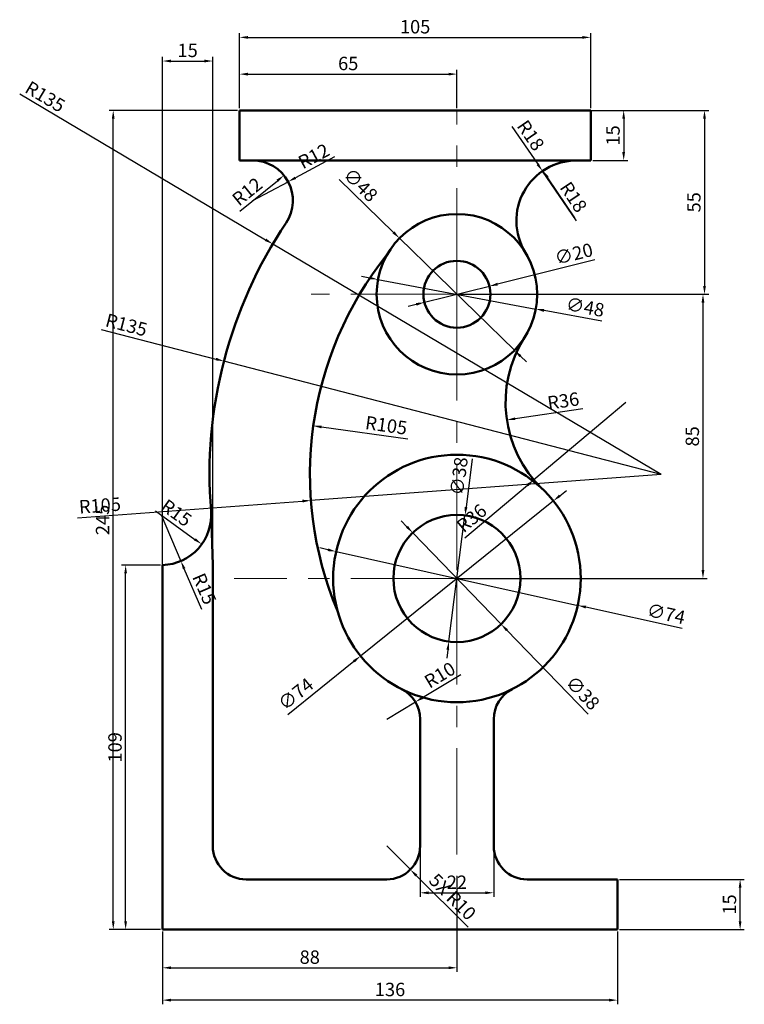
# Model space of a CAD drawing. Units: millimetres. Extents: x 3315 to 3532, y 1569 to 1864.
import ezdxf

# ---------------------------------------------------------------- set-up
doc = ezdxf.new("R2010")
doc.units = ezdxf.units.MM
doc.linetypes.add('CENTER', pattern=[50.8, 31.75, -6.35, 6.35, -6.35])
for name, color, linetype, lineweight in [('M-CNTR', 2, 'CENTER', 18), ('M-DIMS', 120, 'Continuous', 25), ('M-OUTL', 7, 'Continuous', 50)]:
    doc.layers.add(name, color=color, linetype=linetype, lineweight=lineweight)
doc.styles.get("Standard").update_dxf_attribs({"font": 'arial.ttf'})
doc.dimstyles.new('ISO-25', dxfattribs={"dimtxt": 4, "dimasz": 2.5, "dimexe": 1.25, "dimexo": 0.625, "dimtad": 1, "dimtxsty": 'Standard', "dimcen": 2.5, "dimadec": 0, "dimazin": 0, "dimtfac": 1, "dimtmove": 0, "dimatfit": 3, "dimfxl": 1, "dimarcsym": 0})

# ---------------------------------------------------------------- blocks, each defined once
blk = doc.blocks.new('*D1')
at = {"layer": 'Defpoints', "color": 0, "transparency": 16777216}
for p in [(3485.59, 1858.49), (3380.59, 1836.66), (3485.59, 1836.66)]:
    blk.add_point(p, dxfattribs=at)
at = {"layer": 'M-DIMS', "color": 0, "lineweight": -2, "transparency": 16777216}
for p, q in [((3380.59, 1837.28), (3380.59, 1859.74)), ((3383.09, 1858.49), (3483.09, 1858.49)), ((3485.59, 1837.28), (3485.59, 1859.74))]:
    blk.add_line(p, q, dxfattribs=at)
at = {"layer": 'M-DIMS', "color": 0, "transparency": 16777216}
for points in [[(3383.09, 1858.9), (3383.09, 1858.07), (3380.59, 1858.49)], [(3483.09, 1858.9), (3483.09, 1858.07), (3485.59, 1858.49)]]:
    blk.add_solid(points, dxfattribs=at)
at = {"layer": 'M-DIMS', "color": 0, "transparency": 16777216, "insert": (3433.09, 1861.15), "char_height": 4, "attachment_point": 5}
blk.add_mtext('105', dxfattribs=at)
blk = doc.blocks.new('*D2')
at = {"layer": 'Defpoints', "color": 0, "transparency": 16777216}
for p in [(3445.59, 1847.5), (3380.59, 1836.66), (3445.59, 1836.66)]:
    blk.add_point(p, dxfattribs=at)
at = {"layer": 'M-DIMS', "color": 0, "lineweight": -2, "transparency": 16777216}
for p, q in [((3380.59, 1837.28), (3380.59, 1848.75)), ((3383.09, 1847.5), (3443.09, 1847.5)), ((3445.59, 1837.28), (3445.59, 1848.75))]:
    blk.add_line(p, q, dxfattribs=at)
at = {"layer": 'M-DIMS', "color": 0, "transparency": 16777216}
for points in [[(3383.09, 1847.91), (3383.09, 1847.08), (3380.59, 1847.5)], [(3443.09, 1847.91), (3443.09, 1847.08), (3445.59, 1847.5)]]:
    blk.add_solid(points, dxfattribs=at)
at = {"layer": 'M-DIMS', "color": 0, "transparency": 16777216, "insert": (3413.09, 1850.16), "char_height": 4, "attachment_point": 5}
blk.add_mtext('65', dxfattribs=at)
blk = doc.blocks.new('*D3')
at = {"layer": 'Defpoints', "color": 0, "transparency": 16777216}
for p in [(3485.59, 1836.66), (3485.59, 1821.66), (3495.44, 1821.66)]:
    blk.add_point(p, dxfattribs=at)
at = {"layer": 'M-DIMS', "color": 0, "lineweight": -2, "transparency": 16777216}
for p, q in [((3486.21, 1836.66), (3496.69, 1836.66)), ((3495.44, 1834.16), (3495.44, 1824.16)), ((3486.21, 1821.66), (3496.69, 1821.66))]:
    blk.add_line(p, q, dxfattribs=at)
at = {"layer": 'M-DIMS', "color": 0, "transparency": 16777216}
for points in [[(3495.02, 1834.16), (3495.85, 1834.16), (3495.44, 1836.66)], [(3495.02, 1824.16), (3495.85, 1824.16), (3495.44, 1821.66)]]:
    blk.add_solid(points, dxfattribs=at)
at = {"layer": 'M-DIMS', "color": 0, "transparency": 16777216, "insert": (3492.77, 1829.16), "char_height": 4, "attachment_point": 5, "rotation": 90}
blk.add_mtext('15', dxfattribs=at)
blk = doc.blocks.new('*D4')
at = {"layer": 'Defpoints', "color": 0, "transparency": 16777216}
for p in [(3445.59, 1836.66), (3445.59, 1781.66), (3519.6, 1781.66)]:
    blk.add_point(p, dxfattribs=at)
at = {"layer": 'M-DIMS', "color": 0, "lineweight": -2, "transparency": 16777216}
for p, q in [((3446.21, 1836.66), (3520.85, 1836.66)), ((3519.6, 1834.16), (3519.6, 1784.16)), ((3446.21, 1781.66), (3520.85, 1781.66))]:
    blk.add_line(p, q, dxfattribs=at)
at = {"layer": 'M-DIMS', "color": 0, "transparency": 16777216}
for points in [[(3519.18, 1834.16), (3520.02, 1834.16), (3519.6, 1836.66)], [(3519.18, 1784.16), (3520.02, 1784.16), (3519.6, 1781.66)]]:
    blk.add_solid(points, dxfattribs=at)
at = {"layer": 'M-DIMS', "color": 0, "transparency": 16777216, "insert": (3516.94, 1809.16), "char_height": 4, "attachment_point": 5, "rotation": 90}
blk.add_mtext('55', dxfattribs=at)
blk = doc.blocks.new('*D5')
at = {"layer": 'Defpoints', "color": 0, "transparency": 16777216}
for p in [(3445.59, 1781.66), (3445.59, 1696.66), (3519.15, 1696.66)]:
    blk.add_point(p, dxfattribs=at)
at = {"layer": 'M-DIMS', "color": 0, "lineweight": -2, "transparency": 16777216}
for p, q in [((3446.21, 1781.66), (3520.4, 1781.66)), ((3519.15, 1779.16), (3519.15, 1699.16)), ((3446.21, 1696.66), (3520.4, 1696.66))]:
    blk.add_line(p, q, dxfattribs=at)
at = {"layer": 'M-DIMS', "color": 0, "transparency": 16777216}
for points in [[(3518.73, 1779.16), (3519.57, 1779.16), (3519.15, 1781.66)], [(3518.73, 1699.16), (3519.57, 1699.16), (3519.15, 1696.66)]]:
    blk.add_solid(points, dxfattribs=at)
at = {"layer": 'M-DIMS', "color": 0, "transparency": 16777216, "insert": (3516.48, 1739.16), "char_height": 4, "attachment_point": 5, "rotation": 90}
blk.add_mtext('85', dxfattribs=at)
blk = doc.blocks.new('*D6')
at = {"layer": 'Defpoints', "color": 0, "transparency": 16777216}
for p in [(3434.59, 1635.64), (3456.59, 1635.64), (3456.59, 1602.65)]:
    blk.add_point(p, dxfattribs=at)
at = {"layer": 'M-DIMS', "color": 0, "lineweight": -2, "transparency": 16777216}
for p, q in [((3434.59, 1635.01), (3434.59, 1601.4)), ((3456.59, 1635.01), (3456.59, 1601.4)), ((3437.09, 1602.65), (3454.09, 1602.65))]:
    blk.add_line(p, q, dxfattribs=at)
at = {"layer": 'M-DIMS', "color": 0, "transparency": 16777216}
for points in [[(3437.09, 1603.07), (3437.09, 1602.24), (3434.59, 1602.65)], [(3454.09, 1603.07), (3454.09, 1602.24), (3456.59, 1602.65)]]:
    blk.add_solid(points, dxfattribs=at)
at = {"layer": 'M-DIMS', "color": 0, "transparency": 16777216, "insert": (3445.59, 1605.29), "char_height": 4, "attachment_point": 5}
blk.add_mtext('22', dxfattribs=at)
blk = doc.blocks.new('*D7')
at = {"layer": 'Defpoints', "color": 0, "transparency": 16777216}
for p in [(3357.59, 1591.66), (3493.59, 1591.66), (3357.59, 1570.55)]:
    blk.add_point(p, dxfattribs=at)
at = {"layer": 'M-DIMS', "color": 0, "lineweight": -2, "transparency": 16777216}
for p, q in [((3357.59, 1591.03), (3357.59, 1569.3)), ((3493.59, 1591.03), (3493.59, 1569.3)), ((3491.09, 1570.55), (3360.09, 1570.55))]:
    blk.add_line(p, q, dxfattribs=at)
at = {"layer": 'M-DIMS', "color": 0, "transparency": 16777216}
for points in [[(3360.09, 1570.97), (3360.09, 1570.13), (3357.59, 1570.55)], [(3491.09, 1570.97), (3491.09, 1570.13), (3493.59, 1570.55)]]:
    blk.add_solid(points, dxfattribs=at)
at = {"layer": 'M-DIMS', "color": 0, "transparency": 16777216, "insert": (3425.59, 1573.22), "char_height": 4, "attachment_point": 5}
blk.add_mtext('136', dxfattribs=at)
blk = doc.blocks.new('*D8')
at = {"layer": 'Defpoints', "color": 0, "transparency": 16777216}
for p in [(3445.59, 1608.3), (3357.59, 1591.66), (3445.59, 1580.22)]:
    blk.add_point(p, dxfattribs=at)
at = {"layer": 'M-DIMS', "color": 0, "lineweight": -2, "transparency": 16777216}
for p, q in [((3445.59, 1607.67), (3445.59, 1578.97)), ((3357.59, 1591.03), (3357.59, 1578.97)), ((3360.09, 1580.22), (3443.09, 1580.22))]:
    blk.add_line(p, q, dxfattribs=at)
at = {"layer": 'M-DIMS', "color": 0, "transparency": 16777216}
for points in [[(3360.09, 1580.64), (3360.09, 1579.81), (3357.59, 1580.22)], [(3443.09, 1580.64), (3443.09, 1579.81), (3445.59, 1580.22)]]:
    blk.add_solid(points, dxfattribs=at)
at = {"layer": 'M-DIMS', "color": 0, "transparency": 16777216, "insert": (3401.59, 1582.89), "char_height": 4, "attachment_point": 5}
blk.add_mtext('88', dxfattribs=at)
blk = doc.blocks.new('*D9')
at = {"layer": 'Defpoints', "color": 0, "transparency": 16777216}
for p in [(3346.54, 1700.66), (3357.59, 1700.66), (3357.59, 1591.66)]:
    blk.add_point(p, dxfattribs=at)
at = {"layer": 'M-DIMS', "color": 0, "lineweight": -2, "transparency": 16777216}
for p, q in [((3356.96, 1700.66), (3345.29, 1700.66)), ((3346.54, 1594.16), (3346.54, 1698.16)), ((3356.96, 1591.66), (3345.29, 1591.66))]:
    blk.add_line(p, q, dxfattribs=at)
at = {"layer": 'M-DIMS', "color": 0, "transparency": 16777216}
for points in [[(3346.13, 1698.16), (3346.96, 1698.16), (3346.54, 1700.66)], [(3346.13, 1594.16), (3346.96, 1594.16), (3346.54, 1591.66)]]:
    blk.add_solid(points, dxfattribs=at)
at = {"layer": 'M-DIMS', "color": 0, "transparency": 16777216, "insert": (3343.88, 1646.16), "char_height": 4, "attachment_point": 5, "rotation": 90}
blk.add_mtext('109', dxfattribs=at)
blk = doc.blocks.new('*D10')
at = {"layer": 'Defpoints', "color": 0, "transparency": 16777216}
for p in [(3471.33, 1818.6), (3481.36, 1803.66)]:
    blk.add_point(p, dxfattribs=at)
at = {"layer": 'M-DIMS', "color": 0, "lineweight": -2, "transparency": 16777216}
blk.add_line((3480.81, 1804.48), (3472.72, 1816.53), dxfattribs=at)
at = {"layer": 'M-DIMS', "color": 0, "transparency": 16777216}
blk.add_solid([(3473.07, 1816.76), (3472.38, 1816.3), (3471.33, 1818.6)], dxfattribs=at)
at = {"layer": 'M-DIMS', "color": 0, "transparency": 16777216, "insert": (3480.01, 1810.46), "char_height": 4, "attachment_point": 5, "rotation": 303.8767}
blk.add_mtext('R18', dxfattribs=at)
blk = doc.blocks.new('*D11')
at = {"layer": 'Defpoints', "color": 0, "transparency": 16777216}
for p in [(3393.86, 1817.2), (3384.53, 1809.66)]:
    blk.add_point(p, dxfattribs=at)
at = {"layer": 'M-DIMS', "color": 0, "lineweight": -2, "transparency": 16777216}
blk.add_line((3380.68, 1806.54), (3391.92, 1815.63), dxfattribs=at)
at = {"layer": 'M-DIMS', "color": 0, "transparency": 16777216}
blk.add_solid([(3391.66, 1815.96), (3392.18, 1815.31), (3393.86, 1817.2)], dxfattribs=at)
at = {"layer": 'M-DIMS', "color": 0, "transparency": 16777216, "insert": (3383.21, 1811.97), "char_height": 4, "attachment_point": 5, "rotation": 38.9548}
blk.add_mtext('R12', dxfattribs=at)
blk = doc.blocks.new('*D12')
at = {"layer": 'Defpoints', "color": 0, "transparency": 16777216}
for p in [(3375.94, 1761.65), (3506.63, 1727.79)]:
    blk.add_point(p, dxfattribs=at)
at = {"layer": 'M-DIMS', "color": 0, "lineweight": -2, "transparency": 16777216}
for p, q in [((3339.23, 1771.17), (3373.52, 1762.28)), ((3506.63, 1727.79), (3375.94, 1761.65))]:
    blk.add_line(p, q, dxfattribs=at)
at = {"layer": 'M-DIMS', "color": 0, "transparency": 16777216}
blk.add_solid([(3373.63, 1762.68), (3373.42, 1761.88), (3375.94, 1761.65)], dxfattribs=at)
at = {"layer": 'M-DIMS', "color": 0, "transparency": 16777216, "insert": (3346.65, 1772), "char_height": 4, "attachment_point": 5, "rotation": 345.4735}
blk.add_mtext('R135', dxfattribs=at)
blk = doc.blocks.new('*D13')
at = {"layer": 'Defpoints', "color": 0, "transparency": 16777216}
for p in [(3402.63, 1742.3), (3506.63, 1727.79)]:
    blk.add_point(p, dxfattribs=at)
at = {"layer": 'M-DIMS', "color": 0, "lineweight": -2, "transparency": 16777216}
blk.add_line((3430.93, 1738.36), (3405.11, 1741.96), dxfattribs=at)
at = {"layer": 'M-DIMS', "color": 0, "transparency": 16777216}
blk.add_solid([(3405.17, 1742.37), (3405.05, 1741.55), (3402.63, 1742.3)], dxfattribs=at)
at = {"layer": 'M-DIMS', "color": 0, "transparency": 16777216, "insert": (3424.39, 1741.96), "char_height": 4, "attachment_point": 5, "rotation": 352.055}
blk.add_mtext('R105', dxfattribs=at)
blk = doc.blocks.new('*D14')
at = {"layer": 'Defpoints', "color": 0, "transparency": 16777216}
for p in [(3496.13, 1749.33), (3460.52, 1744.06)]:
    blk.add_point(p, dxfattribs=at)
at = {"layer": 'M-DIMS', "color": 0, "lineweight": -2, "transparency": 16777216}
blk.add_line((3483.19, 1747.41), (3462.99, 1744.42), dxfattribs=at)
at = {"layer": 'M-DIMS', "color": 0, "transparency": 16777216}
blk.add_solid([(3462.93, 1744.84), (3463.05, 1744.01), (3460.52, 1744.06)], dxfattribs=at)
at = {"layer": 'M-DIMS', "color": 0, "transparency": 16777216, "insert": (3477.45, 1749.26), "char_height": 4, "attachment_point": 5, "rotation": 8.4211}
blk.add_mtext('R36', dxfattribs=at)
blk = doc.blocks.new('*D15')
at = {"layer": 'Defpoints', "color": 0, "transparency": 16777216}
for p in [(3433.18, 1659.73), (3424.59, 1654.61)]:
    blk.add_point(p, dxfattribs=at)
at = {"layer": 'M-DIMS', "color": 0, "lineweight": -2, "transparency": 16777216}
for p, q in [((3446.74, 1667.82), (3435.32, 1661.01)), ((3424.59, 1654.61), (3433.18, 1659.73))]:
    blk.add_line(p, q, dxfattribs=at)
at = {"layer": 'M-DIMS', "color": 0, "transparency": 16777216}
blk.add_solid([(3435.11, 1661.37), (3435.54, 1660.65), (3433.18, 1659.73)], dxfattribs=at)
at = {"layer": 'M-DIMS', "color": 0, "transparency": 16777216, "insert": (3440.74, 1667.35), "char_height": 4, "attachment_point": 5, "rotation": 30.7966}
blk.add_mtext('R10', dxfattribs=at)
blk = doc.blocks.new('*D16')
at = {"layer": 'Defpoints', "color": 0, "transparency": 16777216}
for p in [(3357.12, 1715.66), (3369.3, 1706.9)]:
    blk.add_point(p, dxfattribs=at)
at = {"layer": 'M-DIMS', "color": 0, "lineweight": -2, "transparency": 16777216}
blk.add_line((3355.46, 1716.85), (3367.27, 1708.36), dxfattribs=at)
at = {"layer": 'M-DIMS', "color": 0, "transparency": 16777216}
blk.add_solid([(3367.51, 1708.7), (3367.02, 1708.02), (3369.3, 1706.9)], dxfattribs=at)
at = {"layer": 'M-DIMS', "color": 0, "transparency": 16777216, "insert": (3361.42, 1715.85), "char_height": 4, "attachment_point": 5, "rotation": 324.2811}
blk.add_mtext('R15', dxfattribs=at)
blk = doc.blocks.new('*D17')
at = {"layer": 'Defpoints', "color": 0, "transparency": 16777216}
for p in [(3428.41, 1798.42), (3462.76, 1764.9)]:
    blk.add_point(p, dxfattribs=at)
at = {"layer": 'M-DIMS', "color": 0, "lineweight": -2, "transparency": 16777216}
for p, q in [((3410.42, 1815.97), (3426.62, 1800.17)), ((3462.76, 1764.9), (3428.41, 1798.42)), ((3464.55, 1763.15), (3466.34, 1761.41))]:
    blk.add_line(p, q, dxfattribs=at)
at = {"layer": 'M-DIMS', "color": 0, "transparency": 16777216}
for points in [[(3426.91, 1800.46), (3426.33, 1799.87), (3428.41, 1798.42)], [(3464.84, 1763.45), (3464.26, 1762.85), (3462.76, 1764.9)]]:
    blk.add_solid(points, dxfattribs=at)
at = {"layer": 'M-DIMS', "color": 0, "transparency": 16777216, "insert": (3416.42, 1814), "char_height": 4, "attachment_point": 5, "rotation": 315.7036}
blk.add_mtext('∅48', dxfattribs=at)
blk = doc.blocks.new('*D18')
at = {"layer": 'Defpoints', "color": 0, "transparency": 16777216}
for p in [(3455.29, 1784.07), (3435.88, 1779.25)]:
    blk.add_point(p, dxfattribs=at)
at = {"layer": 'M-DIMS', "color": 0, "lineweight": -2, "transparency": 16777216}
for p, q in [((3486.81, 1791.91), (3457.72, 1784.67)), ((3435.88, 1779.25), (3455.29, 1784.07)), ((3433.45, 1778.64), (3431.03, 1778.04))]:
    blk.add_line(p, q, dxfattribs=at)
at = {"layer": 'M-DIMS', "color": 0, "transparency": 16777216}
for points in [[(3457.62, 1785.08), (3457.82, 1784.27), (3455.29, 1784.07)], [(3433.35, 1779.05), (3433.56, 1778.24), (3435.88, 1779.25)]]:
    blk.add_solid(points, dxfattribs=at)
at = {"layer": 'M-DIMS', "color": 0, "transparency": 16777216, "insert": (3480.64, 1793.24), "char_height": 4, "attachment_point": 5, "rotation": 13.962}
blk.add_mtext('∅20', dxfattribs=at)
blk = doc.blocks.new('*D19')
at = {"layer": 'Defpoints', "color": 0, "transparency": 16777216}
for p in [(3432.38, 1710.32), (3458.79, 1682.99)]:
    blk.add_point(p, dxfattribs=at)
at = {"layer": 'M-DIMS', "color": 0, "lineweight": -2, "transparency": 16777216}
for p, q in [((3430.65, 1712.12), (3428.91, 1713.92)), ((3432.38, 1710.32), (3458.79, 1682.99)), ((3484.79, 1656.07), (3460.52, 1681.2))]:
    blk.add_line(p, q, dxfattribs=at)
at = {"layer": 'M-DIMS', "color": 0, "transparency": 16777216}
for points in [[(3430.95, 1712.41), (3430.35, 1711.83), (3432.38, 1710.32)], [(3460.82, 1681.49), (3460.22, 1680.91), (3458.79, 1682.99)]]:
    blk.add_solid(points, dxfattribs=at)
at = {"layer": 'M-DIMS', "color": 0, "transparency": 16777216, "insert": (3482.85, 1662.08), "char_height": 4, "attachment_point": 5, "rotation": 314.0096}
blk.add_mtext('∅38', dxfattribs=at)
blk = doc.blocks.new('*D20')
at = {"layer": 'Defpoints', "color": 0, "transparency": 16777216}
for p in [(3409.47, 1704.7), (3481.7, 1688.62)]:
    blk.add_point(p, dxfattribs=at)
at = {"layer": 'M-DIMS', "color": 0, "lineweight": -2, "transparency": 16777216}
for p, q in [((3407.03, 1705.24), (3404.59, 1705.79)), ((3409.47, 1704.7), (3481.7, 1688.62)), ((3512.93, 1681.66), (3484.14, 1688.07))]:
    blk.add_line(p, q, dxfattribs=at)
at = {"layer": 'M-DIMS', "color": 0, "transparency": 16777216}
for points in [[(3407.12, 1705.65), (3406.94, 1704.84), (3409.47, 1704.7)], [(3484.23, 1688.48), (3484.05, 1687.67), (3481.7, 1688.62)]]:
    blk.add_solid(points, dxfattribs=at)
at = {"layer": 'M-DIMS', "color": 0, "transparency": 16777216, "insert": (3508.01, 1685.61), "char_height": 4, "attachment_point": 5, "rotation": 347.4467}
blk.add_mtext('∅74', dxfattribs=at)
blk = doc.blocks.new('*D21')
at = {"layer": 'Defpoints', "color": 0, "transparency": 16777216}
for p in [(3342.84, 1836.66), (3380.59, 1836.66), (3357.59, 1591.66)]:
    blk.add_point(p, dxfattribs=at)
at = {"layer": 'M-DIMS', "color": 0, "lineweight": -2, "transparency": 16777216}
for p, q in [((3379.96, 1836.66), (3341.59, 1836.66)), ((3342.84, 1594.16), (3342.84, 1834.16)), ((3356.96, 1591.66), (3341.59, 1591.66))]:
    blk.add_line(p, q, dxfattribs=at)
at = {"layer": 'M-DIMS', "color": 0, "transparency": 16777216}
for points in [[(3342.42, 1834.16), (3343.25, 1834.16), (3342.84, 1836.66)], [(3342.42, 1594.16), (3343.25, 1594.16), (3342.84, 1591.66)]]:
    blk.add_solid(points, dxfattribs=at)
at = {"layer": 'M-DIMS', "color": 0, "transparency": 16777216, "insert": (3340.17, 1714.16), "char_height": 4, "attachment_point": 5, "rotation": 90}
blk.add_mtext('245', dxfattribs=at)
blk = doc.blocks.new('*D22')
at = {"layer": 'Defpoints', "color": 0, "transparency": 16777216}
for p in [(3493.59, 1606.66), (3530.25, 1606.66), (3493.59, 1591.66)]:
    blk.add_point(p, dxfattribs=at)
at = {"layer": 'M-DIMS', "color": 0, "lineweight": -2, "transparency": 16777216}
for p, q in [((3494.21, 1606.66), (3531.5, 1606.66)), ((3530.25, 1594.16), (3530.25, 1604.16)), ((3494.21, 1591.66), (3531.5, 1591.66))]:
    blk.add_line(p, q, dxfattribs=at)
at = {"layer": 'M-DIMS', "color": 0, "transparency": 16777216}
for points in [[(3529.83, 1604.16), (3530.67, 1604.16), (3530.25, 1606.66)], [(3529.83, 1594.16), (3530.67, 1594.16), (3530.25, 1591.66)]]:
    blk.add_solid(points, dxfattribs=at)
at = {"layer": 'M-DIMS', "color": 0, "transparency": 16777216, "insert": (3527.58, 1599.16), "char_height": 4, "attachment_point": 5, "rotation": 90}
blk.add_mtext('15', dxfattribs=at)
blk = doc.blocks.new('*D23')
at = {"layer": 'Defpoints', "color": 0, "transparency": 16777216}
for p in [(3372.59, 1851.41), (3372.59, 1616.66), (3357.59, 1591.66)]:
    blk.add_point(p, dxfattribs=at)
at = {"layer": 'M-DIMS', "color": 0, "lineweight": -2, "transparency": 16777216}
for p, q in [((3357.59, 1592.28), (3357.59, 1852.66)), ((3372.59, 1617.28), (3372.59, 1852.66)), ((3360.09, 1851.41), (3370.09, 1851.41))]:
    blk.add_line(p, q, dxfattribs=at)
at = {"layer": 'M-DIMS', "color": 0, "transparency": 16777216}
for points in [[(3360.09, 1851.83), (3360.09, 1850.99), (3357.59, 1851.41)], [(3370.09, 1851.83), (3370.09, 1850.99), (3372.59, 1851.41)]]:
    blk.add_solid(points, dxfattribs=at)
at = {"layer": 'M-DIMS', "color": 0, "transparency": 16777216, "insert": (3365.09, 1854.08), "char_height": 4, "attachment_point": 5}
blk.add_mtext('15', dxfattribs=at)
blk = doc.blocks.new('*D24')
at = {"layer": 'Defpoints', "color": 0, "transparency": 16777216}
for p in [(3474.41, 1719.85), (3416.76, 1673.47)]:
    blk.add_point(p, dxfattribs=at)
at = {"layer": 'M-DIMS', "color": 0, "lineweight": -2, "transparency": 16777216}
for p, q in [((3476.36, 1721.42), (3478.31, 1722.99)), ((3474.41, 1719.85), (3416.76, 1673.47)), ((3395.05, 1656), (3414.81, 1671.9))]:
    blk.add_line(p, q, dxfattribs=at)
at = {"layer": 'M-DIMS', "color": 0, "transparency": 16777216}
for points in [[(3476.1, 1721.74), (3476.62, 1721.09), (3474.41, 1719.85)], [(3414.55, 1672.22), (3415.07, 1671.57), (3416.76, 1673.47)]]:
    blk.add_solid(points, dxfattribs=at)
at = {"layer": 'M-DIMS', "color": 0, "transparency": 16777216, "insert": (3397.72, 1661.71), "char_height": 4, "attachment_point": 5, "rotation": 38.8177}
blk.add_mtext('∅74', dxfattribs=at)
blk = doc.blocks.new('*D25')
at = {"layer": 'Defpoints', "color": 0, "transparency": 16777216}
for p in [(3448, 1715.5), (3443.17, 1677.81)]:
    blk.add_point(p, dxfattribs=at)
at = {"layer": 'M-DIMS', "color": 0, "lineweight": -2, "transparency": 16777216}
for p, q in [((3450.17, 1732.44), (3448.32, 1717.98)), ((3443.17, 1677.81), (3448, 1715.5)), ((3442.85, 1675.33), (3442.53, 1672.85))]:
    blk.add_line(p, q, dxfattribs=at)
at = {"layer": 'M-DIMS', "color": 0, "transparency": 16777216}
for points in [[(3447.91, 1718.04), (3448.73, 1717.93), (3448, 1715.5)], [(3442.44, 1675.39), (3443.27, 1675.28), (3443.17, 1677.81)]]:
    blk.add_solid(points, dxfattribs=at)
at = {"layer": 'M-DIMS', "color": 0, "transparency": 16777216, "insert": (3446.69, 1727.17), "char_height": 4, "attachment_point": 5, "rotation": 82.6975}
blk.add_mtext('∅38', dxfattribs=at)
blk = doc.blocks.new('*D26')
at = {"layer": 'Defpoints', "color": 0, "transparency": 16777216}
for p in [(3421.99, 1786.06), (3469.18, 1777.25)]:
    blk.add_point(p, dxfattribs=at)
at = {"layer": 'M-DIMS', "color": 0, "lineweight": -2, "transparency": 16777216}
for p, q in [((3419.54, 1786.52), (3417.08, 1786.98)), ((3421.99, 1786.06), (3469.18, 1777.25)), ((3488.91, 1773.57), (3471.64, 1776.8))]:
    blk.add_line(p, q, dxfattribs=at)
at = {"layer": 'M-DIMS', "color": 0, "transparency": 16777216}
for points in [[(3419.61, 1786.93), (3419.46, 1786.11), (3421.99, 1786.06)], [(3471.71, 1777.2), (3471.56, 1776.39), (3469.18, 1777.25)]]:
    blk.add_solid(points, dxfattribs=at)
at = {"layer": 'M-DIMS', "color": 0, "transparency": 16777216, "insert": (3483.84, 1777.34), "char_height": 4, "attachment_point": 5, "rotation": 349.4246}
blk.add_mtext('∅48', dxfattribs=at)
blk = doc.blocks.new('*D27')
at = {"layer": 'Defpoints', "color": 0, "transparency": 16777216}
for p in [(3471.15, 1818.48), (3481.36, 1803.66)]:
    blk.add_point(p, dxfattribs=at)
at = {"layer": 'M-DIMS', "color": 0, "lineweight": -2, "transparency": 16777216}
for p, q in [((3461.96, 1831.83), (3469.73, 1820.54)), ((3481.36, 1803.66), (3471.15, 1818.48))]:
    blk.add_line(p, q, dxfattribs=at)
at = {"layer": 'M-DIMS', "color": 0, "transparency": 16777216}
blk.add_solid([(3470.08, 1820.78), (3469.39, 1820.3), (3471.15, 1818.48)], dxfattribs=at)
at = {"layer": 'M-DIMS', "color": 0, "transparency": 16777216, "insert": (3467.22, 1828.89), "char_height": 4, "attachment_point": 5, "rotation": 304.565}
blk.add_mtext('R18', dxfattribs=at)
blk = doc.blocks.new('*D28')
at = {"layer": 'Defpoints', "color": 0, "transparency": 16777216}
for p in [(3395.12, 1815.31), (3384.53, 1809.66)]:
    blk.add_point(p, dxfattribs=at)
at = {"layer": 'M-DIMS', "color": 0, "lineweight": -2, "transparency": 16777216}
for p, q in [((3409.03, 1822.73), (3397.33, 1816.48)), ((3384.53, 1809.66), (3395.12, 1815.31))]:
    blk.add_line(p, q, dxfattribs=at)
at = {"layer": 'M-DIMS', "color": 0, "transparency": 16777216}
blk.add_solid([(3397.13, 1816.85), (3397.52, 1816.12), (3395.12, 1815.31)], dxfattribs=at)
at = {"layer": 'M-DIMS', "color": 0, "transparency": 16777216, "insert": (3403.04, 1822.52), "char_height": 4, "attachment_point": 5, "rotation": 28.0775}
blk.add_mtext('R12', dxfattribs=at)
blk = doc.blocks.new('*D29')
at = {"layer": 'Defpoints', "color": 0, "transparency": 16777216}
for p in [(3424.59, 1616.66), (3431.66, 1609.59)]:
    blk.add_point(p, dxfattribs=at)
at = {"layer": 'M-DIMS', "color": 0, "lineweight": -2, "transparency": 16777216}
for p, q in [((3424.59, 1616.66), (3431.66, 1609.59)), ((3448.9, 1592.34), (3433.42, 1607.82))]:
    blk.add_line(p, q, dxfattribs=at)
at = {"layer": 'M-DIMS', "color": 0, "transparency": 16777216}
blk.add_solid([(3433.72, 1608.12), (3433.13, 1607.53), (3431.66, 1609.59)], dxfattribs=at)
at = {"layer": 'M-DIMS', "color": 0, "transparency": 16777216, "insert": (3443.93, 1601.08), "char_height": 4, "attachment_point": 5, "rotation": 315.0025}
blk.add_mtext('5X R10', dxfattribs=at)
blk = doc.blocks.new('*D30')
at = {"layer": 'Defpoints', "color": 0, "transparency": 16777216}
for p in [(3390.53, 1796.69), (3506.63, 1727.79)]:
    blk.add_point(p, dxfattribs=at)
at = {"layer": 'M-DIMS', "color": 0, "lineweight": -2, "transparency": 16777216}
for p, q in [((3314.87, 1841.58), (3388.38, 1797.96)), ((3506.63, 1727.79), (3390.53, 1796.69))]:
    blk.add_line(p, q, dxfattribs=at)
at = {"layer": 'M-DIMS', "color": 0, "transparency": 16777216}
blk.add_solid([(3388.59, 1798.32), (3388.17, 1797.6), (3390.53, 1796.69)], dxfattribs=at)
at = {"layer": 'M-DIMS', "color": 0, "transparency": 16777216, "insert": (3322.23, 1840.32), "char_height": 4, "attachment_point": 5, "rotation": 329.3139}
blk.add_mtext('R135', dxfattribs=at)
blk = doc.blocks.new('*D31')
at = {"layer": 'Defpoints', "color": 0, "transparency": 16777216}
for p in [(3506.63, 1727.79), (3401.92, 1719.99)]:
    blk.add_point(p, dxfattribs=at)
at = {"layer": 'M-DIMS', "color": 0, "lineweight": -2, "transparency": 16777216}
for p, q in [((3506.63, 1727.79), (3401.92, 1719.99)), ((3332.14, 1714.8), (3399.42, 1719.81))]:
    blk.add_line(p, q, dxfattribs=at)
at = {"layer": 'M-DIMS', "color": 0, "transparency": 16777216}
blk.add_solid([(3399.39, 1720.22), (3399.45, 1719.39), (3401.92, 1719.99)], dxfattribs=at)
at = {"layer": 'M-DIMS', "color": 0, "transparency": 16777216, "insert": (3338.89, 1717.98), "char_height": 4, "attachment_point": 5, "rotation": 4.2587}
blk.add_mtext('R105', dxfattribs=at)
blk = doc.blocks.new('*D32')
at = {"layer": 'Defpoints', "color": 0, "transparency": 16777216}
for p in [(3496.13, 1749.33), (3468.57, 1726.16)]:
    blk.add_point(p, dxfattribs=at)
at = {"layer": 'M-DIMS', "color": 0, "lineweight": -2, "transparency": 16777216}
for p, q in [((3496.13, 1749.33), (3468.57, 1726.16)), ((3447.91, 1708.79), (3466.66, 1724.55))]:
    blk.add_line(p, q, dxfattribs=at)
at = {"layer": 'M-DIMS', "color": 0, "transparency": 16777216}
blk.add_solid([(3466.39, 1724.87), (3466.93, 1724.24), (3468.57, 1726.16)], dxfattribs=at)
at = {"layer": 'M-DIMS', "color": 0, "transparency": 16777216, "insert": (3450.32, 1714.31), "char_height": 4, "attachment_point": 5, "rotation": 40.0542}
blk.add_mtext('R36', dxfattribs=at)
blk = doc.blocks.new('*D33')
at = {"layer": 'Defpoints', "color": 0, "transparency": 16777216}
for p in [(3357.12, 1715.66), (3363.05, 1701.88)]:
    blk.add_point(p, dxfattribs=at)
at = {"layer": 'M-DIMS', "color": 0, "lineweight": -2, "transparency": 16777216}
for p, q in [((3357.12, 1715.66), (3363.05, 1701.88)), ((3369.32, 1687.34), (3364.04, 1699.59))]:
    blk.add_line(p, q, dxfattribs=at)
at = {"layer": 'M-DIMS', "color": 0, "transparency": 16777216}
blk.add_solid([(3364.42, 1699.75), (3363.66, 1699.42), (3363.05, 1701.88)], dxfattribs=at)
at = {"layer": 'M-DIMS', "color": 0, "transparency": 16777216, "insert": (3369.62, 1693.37), "char_height": 4, "attachment_point": 5, "rotation": 293.3012}
blk.add_mtext('R15', dxfattribs=at)

msp = doc.modelspace()

# ---------------------------------------------------------------- linework, layer by layer
at = {"layer": 'M-CNTR'}
for p, q in [((3445.586, 1781.659), (3445.586, 1836.659)), ((3445.586, 1781.659), (3402.048, 1781.659)), ((3445.586, 1781.659), (3445.586, 1696.659)), ((3445.586, 1781.659), (3480.697, 1781.659)), ((3445.586, 1696.659), (3378.995, 1696.659)), ((3445.586, 1696.659), (3445.586, 1606.659)), ((3445.586, 1696.659), (3515.501, 1696.659))]:
    msp.add_line(p, q, dxfattribs=at)
at = {"layer": 'M-OUTL'}
for p, q in [((3445.586, 1836.659), (3380.586, 1836.659)), ((3380.586, 1836.659), (3380.586, 1821.659)), ((3485.586, 1836.659), (3445.586, 1836.659)), ((3485.586, 1821.659), (3485.586, 1836.659)), ((3380.586, 1821.659), (3384.533, 1821.659)), ((3384.533, 1821.659), (3481.363, 1821.659)), ((3481.363, 1821.659), (3485.586, 1821.659)), ((3372.586, 1700.659), (3372.068, 1716.872)), ((3357.586, 1700.666), (3357.586, 1591.659)), ((3357.586, 1591.659), (3357.586, 1700.659)), ((3372.586, 1700.659), (3372.586, 1616.659)), ((3434.586, 1654.611), (3434.586, 1616.659)), ((3456.586, 1654.611), (3456.586, 1616.659)), ((3424.586, 1606.659), (3382.586, 1606.659)), ((3493.586, 1606.659), (3466.586, 1606.659)), ((3493.586, 1591.659), (3493.586, 1606.659)), ((3357.586, 1591.659), (3493.586, 1591.659))]:
    msp.add_line(p, q, dxfattribs=at)
for centre, radius in [((3445.586, 1781.659), 24), ((3445.586, 1781.659), 10), ((3445.586, 1696.659), 37), ((3445.586, 1696.659), 19)]:
    msp.add_circle(centre, radius, dxfattribs=at)
for centre, radius, start, end in [((3384.533, 1809.659), 12, 326.15669, 90), ((3481.363, 1803.659), 18, 90, 211.58814), ((3506.626, 1727.791), 135, 146.15669, 184.63924), ((3506.626, 1727.791), 105, 141.3106, 202.8425), ((3496.131, 1749.329), 36, 147.39641, 226.1797), ((3357.117, 1715.659), 15, 271.78911, 4.63924), ((3424.586, 1654.611), 10, 0, 63.4609), ((3466.586, 1654.611), 10, 116.5391, 180), ((3382.586, 1616.659), 10, 180, 270), ((3424.586, 1616.659), 10, 270, 0), ((3466.586, 1616.659), 10, 180, 270)]:
    msp.add_arc(centre, radius, start, end, dxfattribs=at)

# ---------------------------------------------------------------- dimensions: what is measured, and where the dimension line sits
at = {"layer": 'M-DIMS'}
for base, p1, p2, override, picture, middle in [((3485.586, 1858.485), (3380.586, 1836.659), (3485.586, 1836.659), {"dimclrd": 0, "dimclre": 0, "dimclrt": 0}, '*D1', (3433.086, 1861.152)), ((3372.586, 1851.409), (3357.586, 1591.659), (3372.586, 1616.659), {"dimdec": 0, "dimlfac": 1, "dimrnd": 0, "dimzin": 0, "dimdsep": 46, "dimlunit": 2}, '*D23', (3365.086, 1854.076)), ((3445.586, 1847.497), (3380.586, 1836.659), (3445.586, 1836.659), {"dimclrd": 0, "dimclre": 0, "dimclrt": 0}, '*D2', (3413.086, 1850.164)), ((3456.586, 1602.652), (3434.586, 1635.635), (3456.586, 1635.635), {"dimclrd": 0, "dimclre": 0, "dimclrt": 0}, '*D6', (3445.586, 1605.285)), ((3445.586, 1580.222), (3357.586, 1591.659), (3445.586, 1608.297), {"dimclrd": 0, "dimclre": 0, "dimclrt": 0}, '*D8', (3401.586, 1582.889)), ((3357.586, 1570.551), (3493.586, 1591.659), (3357.586, 1591.659), {"dimclrd": 0, "dimclre": 0, "dimclrt": 0}, '*D7', (3425.586, 1573.22))]:
    dim = msp.add_linear_dim(base=base, p1=p1, p2=p2, dimstyle='ISO-25', override=override, dxfattribs=at)
    dim.commit()
    dim.dimension.update_dxf_attribs({"geometry": picture, "text_midpoint": middle})
for center, mpoint, override, picture, middle in [((3506.626, 1727.791), (3390.529, 1796.686), {"dimdec": 0, "dimlfac": 1, "dimrnd": 0, "dimzin": 0, "dimdsep": 46, "dimlunit": 2}, '*D30', (3320.871, 1838.023)), ((3481.363, 1803.659), (3471.151, 1818.482), {"dimdec": 0, "dimlfac": 1, "dimrnd": 0, "dimzin": 0, "dimdsep": 46, "dimlunit": 2}, '*D27', (3465.023, 1827.375)), ((3384.533, 1809.659), (3393.865, 1817.203), {"dimclrd": 0, "dimclre": 0, "dimclrt": 0}, '*D11', (3384.865, 1809.927)), ((3481.363, 1803.659), (3471.329, 1818.603), {"dimclrd": 0, "dimclre": 0, "dimclrt": 0}, '*D10', (3477.797, 1808.969)), ((3506.626, 1727.791), (3375.942, 1761.653), {"dimclrd": 0, "dimclre": 0, "dimclrt": 0}, '*D12', (3345.979, 1769.416)), ((3496.131, 1749.329), (3460.519, 1744.057), {"dimclrd": 0, "dimclre": 0, "dimclrt": 0}, '*D14', (3477.842, 1746.622)), ((3496.131, 1749.329), (3468.575, 1726.163), {"dimdec": 0, "dimlfac": 1, "dimrnd": 0, "dimzin": 0, "dimdsep": 46, "dimlunit": 2}, '*D32', (3452.042, 1712.263)), ((3506.626, 1727.791), (3402.634, 1742.304), {"dimclrd": 0, "dimclre": 0, "dimclrt": 0}, '*D13', (3424.022, 1739.319)), ((3506.626, 1727.791), (3401.916, 1719.994), {"dimdec": 0, "dimlfac": 1, "dimrnd": 0, "dimzin": 0, "dimdsep": 46, "dimlunit": 2}, '*D31', (3339.09, 1715.315)), ((3357.117, 1715.659), (3369.296, 1706.902), {"dimclrd": 0, "dimclre": 0, "dimclrt": 0}, '*D16', (3359.863, 1713.684))]:
    dim = msp.add_radius_dim(center=center, mpoint=mpoint, dimstyle='ISO-25', override=override, dxfattribs=at)
    dim.commit()
    dim.dimension.update_dxf_attribs({"geometry": picture, "text_midpoint": middle, "dimtype": 164})
for base, p1, p2, override, picture, middle in [((3342.836, 1836.659), (3357.586, 1591.659), (3380.586, 1836.659), {"dimdec": 0, "dimlfac": 1, "dimrnd": 0, "dimzin": 0, "dimdsep": 46, "dimlunit": 2}, '*D21', (3340.168, 1714.159)), ((3519.601, 1781.659), (3445.586, 1836.659), (3445.586, 1781.659), {"dimclrd": 0, "dimclre": 0, "dimclrt": 0}, '*D4', (3516.942, 1809.159)), ((3495.438, 1821.659), (3485.586, 1836.659), (3485.586, 1821.659), {"dimclrd": 0, "dimclre": 0, "dimclrt": 0}, '*D3', (3492.77, 1829.159)), ((3519.151, 1696.659), (3445.586, 1781.659), (3445.586, 1696.659), {"dimclrd": 0, "dimclre": 0, "dimclrt": 0}, '*D5', (3516.484, 1739.159)), ((3346.543, 1700.659), (3357.586, 1591.659), (3357.586, 1700.659), {"dimclrd": 0, "dimclre": 0, "dimclrt": 0}, '*D9', (3343.875, 1646.159)), ((3530.251, 1606.659), (3493.586, 1591.659), (3493.586, 1606.659), {"dimdec": 0, "dimlfac": 1, "dimrnd": 0, "dimzin": 0, "dimdsep": 46, "dimlunit": 2}, '*D22', (3527.584, 1599.159))]:
    dim = msp.add_linear_dim(base=base, p1=p1, p2=p2, angle=90, dimstyle='ISO-25', override=override, dxfattribs=at)
    dim.commit()
    dim.dimension.update_dxf_attribs({"geometry": picture, "text_midpoint": middle})
for center, mpoint, override, picture, middle in [((3384.533, 1809.659), (3395.121, 1815.307), {"dimdec": 0, "dimlfac": 1, "dimrnd": 0, "dimzin": 0, "dimdsep": 46, "dimlunit": 2}, '*D28', (3403.043, 1822.517)), ((3357.117, 1715.659), (3363.051, 1701.882), {"dimdec": 0, "dimlfac": 1, "dimrnd": 0, "dimzin": 0, "dimdsep": 46, "dimlunit": 2}, '*D33', (3369.622, 1693.368)), ((3424.586, 1654.611), (3433.175, 1659.731), {"dimclrd": 0, "dimclre": 0, "dimclrt": 0}, '*D15', (3440.741, 1667.346))]:
    dim = msp.add_radius_dim(center=center, mpoint=mpoint, dimstyle='ISO-25', override=override, dxfattribs=at)
    dim.commit()
    dim.dimension.update_dxf_attribs({"geometry": picture, "text_midpoint": middle})
for p1, p2, override, picture, middle in [((3462.763, 1764.898), (3428.408, 1798.42), {"dimclrd": 0, "dimclre": 0, "dimclrt": 0}, '*D17', (3414.475, 1812.015)), ((3435.881, 1779.246), (3455.29, 1784.072), {"dimclrd": 0, "dimclre": 0, "dimclrt": 0}, '*D18', (3481.314, 1790.542)), ((3421.993, 1786.064), (3469.178, 1777.254), {"dimdec": 0, "dimlfac": 1, "dimrnd": 0, "dimzin": 0, "dimdsep": 46, "dimlunit": 2}, '*D26', (3483.333, 1774.611)), ((3443.17, 1677.813), (3448.001, 1715.505), {"dimdec": 0, "dimlfac": 1, "dimrnd": 0, "dimzin": 0, "dimdsep": 46, "dimlunit": 2}, '*D25', (3449.45, 1726.812)), ((3474.414, 1719.852), (3416.757, 1673.466), {"dimdec": 0, "dimlfac": 1, "dimrnd": 0, "dimzin": 0, "dimdsep": 46, "dimlunit": 2}, '*D24', (3399.46, 1659.55)), ((3432.385, 1710.324), (3458.786, 1682.994), {"dimclrd": 0, "dimclre": 0, "dimclrt": 0}, '*D19', (3480.853, 1660.151)), ((3409.47, 1704.701), (3481.701, 1688.617), {"dimclrd": 0, "dimclre": 0, "dimclrt": 0}, '*D20', (3507.408, 1682.893))]:
    dim = msp.add_diameter_dim_2p(p1=p1, p2=p2, dimstyle='ISO-25', override=override, dxfattribs=at)
    dim.commit()
    dim.dimension.update_dxf_attribs({"geometry": picture, "text_midpoint": middle, "dimtype": 163})
dim = msp.add_radius_dim(center=(3424.586, 1616.659), mpoint=(3431.657, 1609.588), text='5X <>', dimstyle='ISO-25', override={"dimdec": 0, "dimlfac": 1, "dimrnd": 0, "dimzin": 0, "dimdsep": 46, "dimlunit": 2}, dxfattribs=at)
dim.commit()
dim.dimension.update_dxf_attribs({"geometry": '*D29', "text_midpoint": (3443.934, 1601.084)})

doc.saveas('drawing.dxf')
